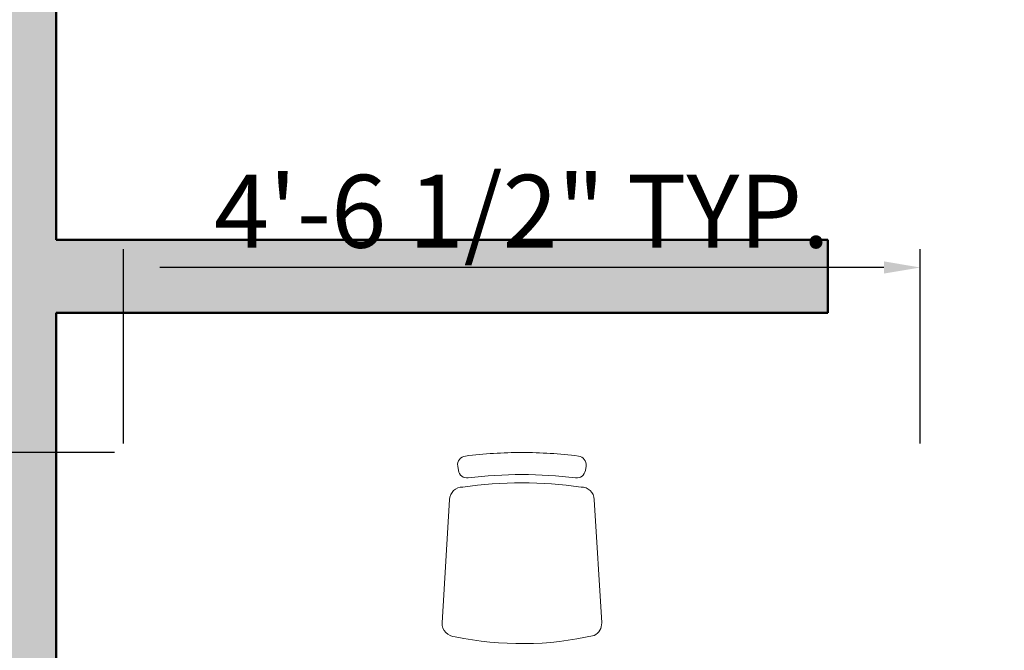
# Model space of a CAD drawing. Units: inches. Extents: x 1734 to 4011, y 1071 to 1891.
# Tile 21 of 27: x 3311 to 3379, y 1723 to 1766. Entities that reach past the tile are written whole.
import ezdxf

# ---------------------------------------------------------------- set-up
doc = ezdxf.new("R2010")
doc.units = ezdxf.units.IN
for name, color, linetype, lineweight in [('A-ANNO-DIMS', 2, 'Continuous', 18), ('A-FURN', 8, 'Continuous', 18), ('A-WALL', 7, 'Continuous', 50), ('A-WALL-PATT', 8, 'Continuous', 13)]:
    doc.layers.add(name, color=color, linetype=linetype, lineweight=lineweight)
doc.styles.get("Standard").update_dxf_attribs({"font": 'arial.ttf'})
doc.dimstyles.new('ISO-25', dxfattribs={"dimtxt": 5, "dimasz": 2.5, "dimexe": 1.25, "dimexo": 0.625, "dimtad": 1, "dimdec": 1, "dimlunit": 3, "dimtxsty": 'Standard', "dimcen": 2.5, "dimclrt": 1, "dimadec": 0, "dimazin": 0, "dimtfac": 1, "dimtdec": 1, "dimtmove": 0, "dimatfit": 3, "dimfxl": 1, "dimarcsym": 0})

# ---------------------------------------------------------------- blocks, each defined once
blk = doc.blocks.new('A$C421907B3')
at = {"ltscale": 0.1}
for points in [[(0.77, 0.0782, -0.399285), (0.74, 0.1067), (0.7231, 0.3861, -0.305593), (0.7404, 0.4148, -0.109362), (1.0554, 0.4176, -0.429301), (1.0853, 0.3861), (1.0684, 0.1067, -0.399285), (1.0384, 0.0782, -0.071734)], [(0.9042, 0.05, 0.030867), (1.0261, 0.0575, -0.408428), (1.0484, 0.0405), (1.0498, 0.0306, -0.419966), (1.0325, 0.0079, -0.030916), (0.9042, 0, -0.030916), (0.7759, 0.0079, -0.419966), (0.7586, 0.0306), (0.76, 0.0405, -0.408428), (0.7823, 0.0575, 0.030867)]]:
    blk.add_lwpolyline(points, format="xyb", close=True, dxfattribs=at)
blk = doc.blocks.new('*D99')
at = {"layer": 'A-ANNO-DIMS', "color": 0, "lineweight": -2, "transparency": 16777216}
for p, q in [((3317.994, 1736.234), (3304.669, 1736.234)), ((3305.919, 1733.734), (3305.919, 1654.07)), ((3317.994, 1651.57), (3304.669, 1651.57)), ((3305.919, 1651.57), (3305.919, 1564.027))]:
    blk.add_line(p, q, dxfattribs=at)
at = {"layer": 'A-ANNO-DIMS', "color": 0, "transparency": 16777216}
for points in [[(3305.503, 1733.734), (3306.336, 1733.734), (3305.919, 1736.234)], [(3305.503, 1654.07), (3306.336, 1654.07), (3305.919, 1651.57)]]:
    blk.add_solid(points, dxfattribs=at)
at = {"layer": 'Defpoints', "color": 0, "transparency": 16777216}
for p in [(3318.619, 1736.234), (3305.919, 1651.57), (3318.619, 1651.57)]:
    blk.add_point(p, dxfattribs=at)
at = {"layer": 'A-ANNO-DIMS', "color": 1, "transparency": 16777216, "insert": (3302.709, 1606.548), "char_height": 5, "attachment_point": 5, "rotation": 90}
blk.add_mtext('DINING SET 7\'-0 1/2" TYP.', dxfattribs=at)
blk = doc.blocks.new('*D100')
at = {"layer": 'A-ANNO-DIMS', "color": 0, "lineweight": -2, "transparency": 16777216}
for p, q in [((3318.619, 1736.859), (3318.619, 1750.183)), ((3373.342, 1736.859), (3373.342, 1750.183)), ((3370.842, 1748.933), (3321.119, 1748.933))]:
    blk.add_line(p, q, dxfattribs=at)
at = {"layer": 'A-ANNO-DIMS', "color": 0, "transparency": 16777216}
for points in [[(3321.119, 1749.35), (3321.119, 1748.516), (3318.619, 1748.933)], [(3370.842, 1749.35), (3370.842, 1748.516), (3373.342, 1748.933)]]:
    blk.add_solid(points, dxfattribs=at)
at = {"layer": 'Defpoints', "color": 0, "transparency": 16777216}
for p in [(3318.619, 1748.933), (3318.619, 1736.234), (3373.342, 1736.234)]:
    blk.add_point(p, dxfattribs=at)
at = {"layer": 'A-ANNO-DIMS', "color": 1, "transparency": 16777216, "insert": (3345.98, 1752.143), "char_height": 5, "attachment_point": 5}
blk.add_mtext('4\'-6 1/2" TYP.', dxfattribs=at)

msp = doc.modelspace()

# ---------------------------------------------------------------- hatches: boundary and pattern name
at = {"layer": 'A-WALL-PATT'}
h = msp.add_hatch(color=256, dxfattribs=at)
h.dxf.hatch_style = 1
h.paths.add_polyline_path([(3475.994, 1831.819), (3115.994, 1831.819), (3115.994, 1745.819), (3130.994, 1745.819), (3130.994, 1750.819), (3124.994, 1750.819), (3124.994, 1822.819), (3214.994, 1822.819), (3214.994, 1780.819), (3219.994, 1780.819), (3219.994, 1822.819), (3308.994, 1822.819), (3308.994, 1750.819), (3254.994, 1750.819), (3254.994, 1745.819), (3308.994, 1745.819), (3308.994, 1604.819), (3313.994, 1604.819), (3313.994, 1745.819), (3366.994, 1745.819), (3366.994, 1750.819), (3313.994, 1750.819), (3313.994, 1822.819), (3401.994, 1822.819), (3401.994, 1750.819), (3396.994, 1750.819), (3396.994, 1745.819), (3411.994, 1745.819), (3411.994, 1750.819), (3406.994, 1750.819), (3406.994, 1822.819), (3466.994, 1822.819), (3466.994, 1750.819), (3441.994, 1750.819), (3441.994, 1745.819), (3466.994, 1745.819), (3466.994, 1517.819), (3452.494, 1517.819), (3452.494, 1512.819), (3466.994, 1512.819), (3466.994, 1458.819), (3446.494, 1458.819), (3446.494, 1453.819), (3466.994, 1453.819), (3466.994, 1237.819), (3372.994, 1237.819), (3372.994, 1228.819), (3466.994, 1228.819), (3466.994, 1120.819), (3309.994, 1120.819), (3309.994, 1184.819), (3310.994, 1184.819), (3310.994, 1189.819), (3303.994, 1189.819), (3303.994, 1120.819), (3291.994, 1120.819), (3291.994, 1111.819), (3475.994, 1111.819)])
h.paths.add_polyline_path([(3169.994, 1745.819), (3224.994, 1745.819), (3224.994, 1750.819), (3154.994, 1750.819), (3154.994, 1745.819), (3160.994, 1745.819), (3160.994, 1636.819), (3169.994, 1636.819)], flags=17)
h.paths.add_polyline_path([(3169.994, 1588.819), (3160.994, 1588.819), (3160.994, 1559.819), (3313.994, 1559.819), (3313.994, 1568.819), (3308.994, 1568.819), (3308.994, 1564.819), (3169.994, 1564.819)], flags=17)
h.paths.add_polyline_path([(3416.494, 1517.819), (3401.994, 1517.819), (3401.994, 1512.819), (3416.494, 1512.819)], flags=17)
h.paths.add_polyline_path([(3371.994, 1517.819), (3366.994, 1517.819), (3366.994, 1453.819), (3392.494, 1453.819), (3392.494, 1458.819), (3371.994, 1458.819)], flags=17)
h.paths.add_polyline_path([(3258.994, 1529.819), (3160.994, 1529.819), (3160.994, 1494.819), (3169.994, 1494.819), (3169.994, 1524.819), (3253.994, 1524.819), (3253.994, 1520.819), (3258.994, 1520.819)], flags=17)
h.paths.add_polyline_path([(3263.994, 1458.819), (3258.994, 1458.819), (3258.994, 1490.819), (3253.994, 1490.819), (3253.994, 1458.819), (3169.994, 1458.819), (3169.994, 1470.819), (3160.994, 1470.819), (3160.994, 1387.819), (3169.994, 1387.819), (3169.994, 1453.819), (3263.994, 1453.819)], flags=17)
h.paths.add_polyline_path([(3313.994, 1453.819), (3318.994, 1453.819), (3318.994, 1458.819), (3299.994, 1458.819), (3299.994, 1453.819), (3308.994, 1453.819), (3308.994, 1321.819), (3266.494, 1321.819), (3266.494, 1312.819), (3313.994, 1312.819)], flags=17)
h.paths.add_polyline_path([(3212.494, 1321.819), (3169.994, 1321.819), (3169.994, 1339.819), (3160.994, 1339.819), (3160.994, 1312.819), (3212.494, 1312.819)], flags=17)
h.paths.add_polyline_path([(3313.994, 1288.819), (3304.994, 1288.819), (3304.994, 1285.819), (3313.994, 1285.819)], flags=17)
h.paths.add_polyline_path([(3324.994, 1237.819), (3304.994, 1237.819), (3304.994, 1228.819), (3324.994, 1228.819)], flags=17)

# ---------------------------------------------------------------- linework, layer by layer
at = {"layer": 'A-WALL'}
for p, q in [((3313.994, 1750.819), (3313.994, 1822.819)), ((3313.994, 1750.819), (3366.994, 1750.819)), ((3366.994, 1745.819), (3366.994, 1750.819)), ((3313.994, 1745.819), (3366.994, 1745.819)), ((3313.994, 1604.819), (3313.994, 1745.819))]:
    msp.add_line(p, q, dxfattribs=at)

# ---------------------------------------------------------------- block references
at = {"layer": 'A-FURN', "xscale": 30.26057373645948, "yscale": 30.26057373645948, "zscale": 30.26057373645948, "rotation": 180}
msp.add_blockref('A$C421907B3', (3373.342, 1736.234), dxfattribs=at)

# ---------------------------------------------------------------- dimensions: what is measured, and where the dimension line sits
at = {"layer": 'A-ANNO-DIMS'}
for base, p1, p2, angle, text, picture, middle in [((3318.619, 1748.933), (3373.342, 1736.234), (3318.619, 1736.234), 180, '<> TYP.', '*D100', (3345.98, 1752.143)), ((3305.919, 1651.57), (3318.619, 1736.234), (3318.619, 1651.57), 270, 'DINING SET <> TYP.', '*D99', (3302.709, 1606.548))]:
    dim = msp.add_linear_dim(base=base, p1=p1, p2=p2, angle=angle, text=text, dimstyle='ISO-25', override={"dimdec": 1, "dimrnd": 0, "dimzin": 1, "dimlunit": 4, "dimfrac": 2}, dxfattribs=at)
    dim.commit()
    dim.dimension.update_dxf_attribs({"geometry": picture, "text_midpoint": middle})

doc.saveas('drawing.dxf')
